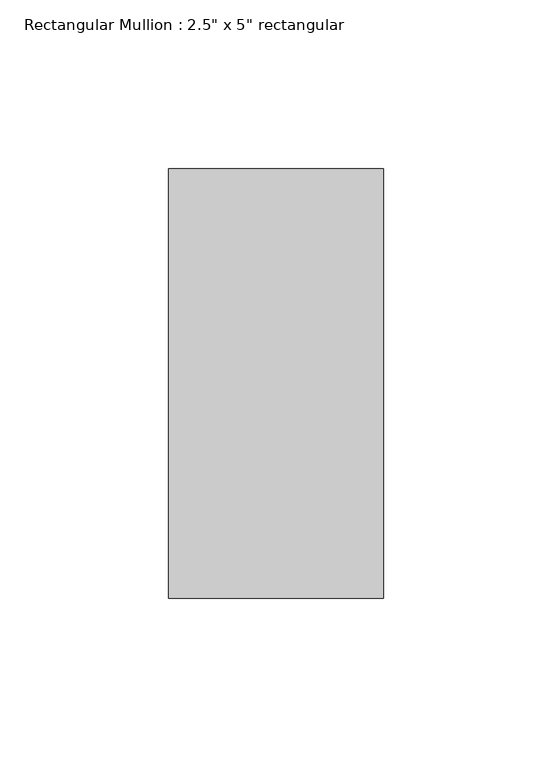
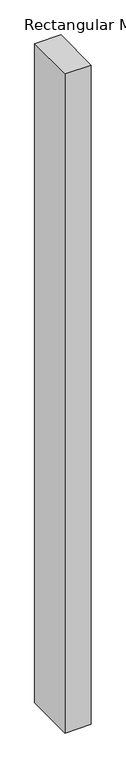
"""IFC4 building model written with IfcOpenShell, lengths in millimetres: member geometry."""

from ifc_helpers import new_model, si_unit, frame, origin, place, context, project, spatial, polyline, outline, extrude, source, transform, mapped, element, save


def member_76c917ad(model_context):
    return source(origin(), model_context, "Body", "SweptSolid", [
        extrude(outline(polyline([(31.75, 63.5), (31.75, -63.5), (-31.75, -63.5), (-31.75, 63.5), (31.75, 63.5)])), frame((0.0, 0.0, -1686.8910355), z_axis=(0.0, 0.0, 1.0), x_axis=(1.0, 0.0, 0.0)), (0.0, 0.0, 1.0), 1686.8910355),
    ])


if __name__ == "__main__":
    model = new_model("IFC4")
    model_context = context("Model", 3, world=origin())
    ifc_project = project(units=[si_unit("LENGTHUNIT", "METRE", prefix="MILLI")], contexts=[model_context])
    site = spatial("IfcSite", under=ifc_project)
    building = spatial("IfcBuilding", under=site)
    placement = place(None, origin())
    member_shape = member_76c917ad(model_context)
    element("IfcMember", 1, ObjectType="Rectangular Mullion : 2.5\" x 5\" rectangular", at=placement, inside=building, context=model_context, shape_type="MappedRepresentation", body=[
        mapped(member_shape, transform((0.0, 0.0, 0.0), x_axis=(1.0, 0.0, 0.0), y_axis=(0.0, 1.0, 0.0), z_axis=(0.0, 0.0, 1.0))),
    ])
    save(model, "model.ifc")

# Revit data of these elements
# Type "Rectangular Mullion : 2.5\" x 5\" rectangular"
#   built-in parameter 1007304 = 0.416667 (stored number, unit not read)
#   built-in parameter 1007301 = 0.104167 (stored number, unit not read)
#   built-in parameter 1007300 = 0.104167 (stored number, unit not read)
# Element 1 (IfcMember, "Rectangular Mullion : 2.5\" x 5\" rectangular")
#   Materials on its faces: "Aluminum"
# Materials
#   "Aluminum": class "Metal", colour RGB 247 247 247, transparency 0, Description = "Aluminum 6061", Cost = 0
